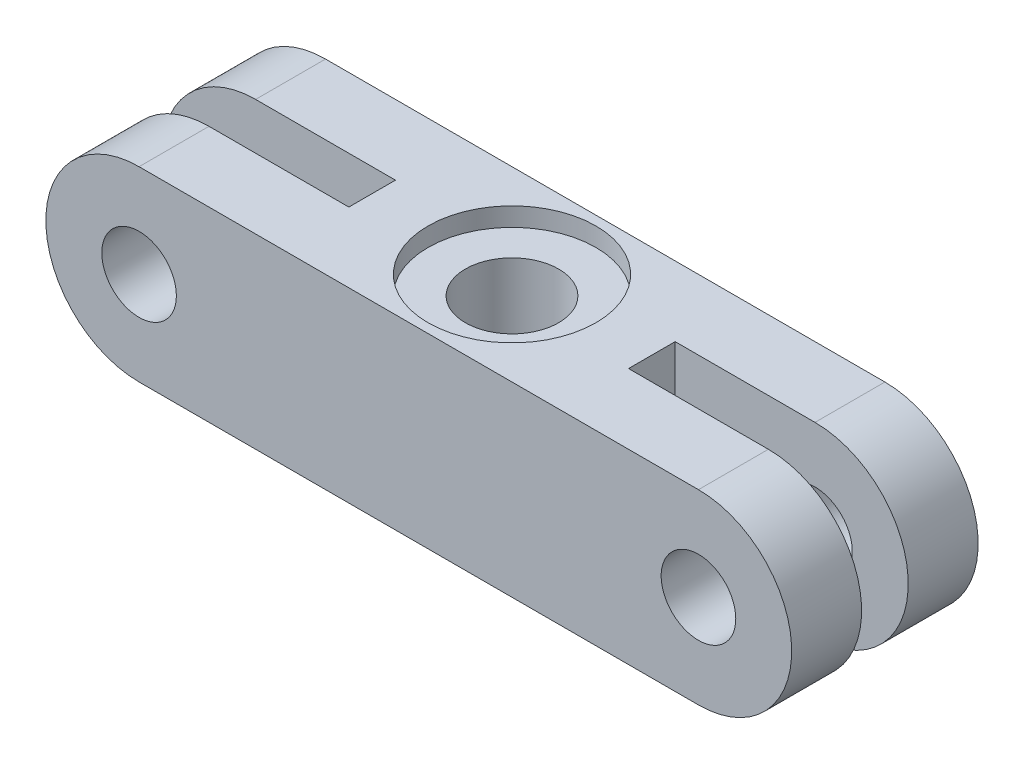
SolidWorks part; units mm, degrees
material "Plain Carbon Steel"
ref_plane "Front Plane" through (0, 0, 0) normal (0, 0, 1) x (1, 0, 0)
ref_plane "Top Plane" through (0, 0, 0) normal (0, 1, 0) x (1, 0, 0)
ref_plane "Right Plane" through (0, 0, 0) normal (1, 0, 0) x (0, 0, -1)
sketch "Link Profile Sketch" plane through (0, 0, 0) normal (0, 0, 1) x (1, 0, 0)
  line L0 (-30, 0) -> (30, 0) construction
  line L1 (-30, 10) -> (30, 10)
  line L2 (-30, -10) -> (30, -10)
  arc A0 (-30, 10) -> (-30, -10) centre (-30, 0) ccw
  arc A1 (30, -10) -> (30, 10) centre (30, 0) ccw
  circle A2 centre (-30, 0) radius 4
  circle A3 centre (30, 0) radius 4
  point P2 (0, 0)
  dimension "D1" = 10
  dimension "D3" = 8
  dimension "D2" = 60
extrude "Link Body" add sketch "Link Profile Sketch" along normal mid plane 20
sketch "End Slots Sketch" plane through (0, 10, 0) normal (0, 1, 0) x (1, 0, 0)
  line L0 (-40, 10) -> (-40, -10) construction
  line L1 (-15, -2.5) -> (-40, -2.5)
  line L2 (-15, -2.5) -> (-15, 2.5)
  line L3 (-15, 2.5) -> (-40, 2.5)
  line L4 (-40, -2.5) -> (-40, 2.5)
  line L5 (-15, -2.5) -> (-40, 2.5) construction
  line L6 (-15, 2.5) -> (-40, -2.5) construction
  line L7 (0, 0) -> (0, 14.1666) construction
  line L8 (15, 2.5) -> (40, -2.5) construction
  line L9 (15, -2.5) -> (40, 2.5) construction
  line L10 (40, -2.5) -> (40, 2.5)
  line L11 (15, 2.5) -> (40, 2.5)
  line L12 (15, -2.5) -> (15, 2.5)
  line L13 (15, -2.5) -> (40, -2.5)
  point P0 (-27.5, 0)
  point P7 (-15, 0)
  point P15 (27.5, 0)
  dimension "D1" = 25
  dimension "D2" = 5
extrude "End Clevis Slots 5mm" cut sketch "End Slots Sketch" against normal through all both
sketch "Centre Hole Sketch" plane through (0, 10, 0) normal (0, 1, 0) x (1, 0, 0)
  circle A0 centre (0, 0) radius 5
  dimension "D1" = 10
extrude "Centre Hole Ø10" cut sketch "Centre Hole Sketch" against normal through all both
sketch "Counterbore Sketch" plane through (0, 10, 0) normal (0, 1, 0) x (1, 0, 0)
  circle A0 centre (0, 0) radius 9
  dimension "D1" = 18
extrude "Counterbore Ø18x2" cut sketch "Counterbore Sketch" against normal blind 2
